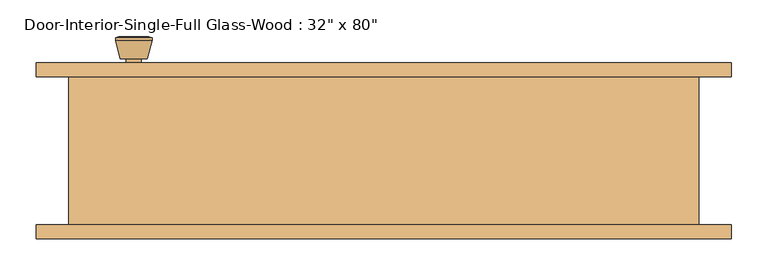
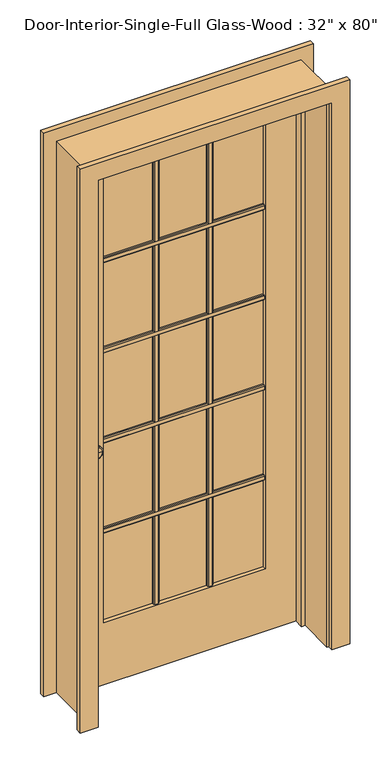
"""IFC4 building model written with IfcOpenShell, lengths in millimetres: door geometry."""

from ifc_helpers import new_model, si_unit, point, frame, frame_2d, origin, place, context, project, spatial, polyline, circle_curve, trimmed, segment, composite_curve, outline, extrude, faceted_brep, source, transform, mapped, element, save
from ifc_brep_helpers import plane_surface, cylinder_surface, revolved_surface, advanced_brep


def door_22967355(model_context):
    return source(origin(), model_context, "Body", "SolidModel", [
        extrude(outline(polyline([(84.455, 1586.23), (90.805, 1586.23), (93.98, 1583.055), (93.98, 1570.355), (90.805, 1567.18), (84.455, 1567.18), (84.455, 1586.23)])), frame((-285.75, 0.0, 0.0), z_axis=(1.0, 0.0, 0.0), x_axis=(0.0, 1.0, 0.0)), (0.0, 0.0, 1.0), 571.5),
        extrude(outline(polyline([(84.455, 1249.9975), (90.805, 1249.9975), (93.98, 1246.8225), (93.98, 1234.1225), (90.805, 1230.9475), (84.455, 1230.9475), (84.455, 1249.9975)])), frame((-285.75, 0.0, 0.0), z_axis=(1.0, 0.0, 0.0), x_axis=(0.0, 1.0, 0.0)), (0.0, 0.0, 1.0), 571.5),
        extrude(outline(polyline([(84.455, 913.765), (90.805, 913.765), (93.98, 910.59), (93.98, 897.89), (90.805, 894.715), (84.455, 894.715), (84.455, 913.765)])), frame((-285.75, 0.0, 0.0), z_axis=(1.0, 0.0, 0.0), x_axis=(0.0, 1.0, 0.0)), (0.0, 0.0, 1.0), 571.5),
        extrude(outline(polyline([(84.455, 577.5325), (90.805, 577.5325), (93.98, 574.3575), (93.98, 561.6575), (90.805, 558.4825), (84.455, 558.4825), (84.455, 577.5325)])), frame((-285.75, 0.0, 0.0), z_axis=(1.0, 0.0, 0.0), x_axis=(0.0, 1.0, 0.0)), (0.0, 0.0, 1.0), 571.5),
        extrude(outline(polyline([(85.725, 84.455), (85.725, 90.805), (88.9, 93.98), (101.6, 93.98), (104.775, 90.805), (104.775, 84.455), (85.725, 84.455)])), frame((0.0, 0.0, 231.775), z_axis=(0.0, 0.0, 1.0), x_axis=(1.0, 0.0, 0.0)), (0.0, 0.0, 1.0), 1681.1625),
        extrude(outline(polyline([(-104.775, 84.455), (-104.775, 90.805), (-101.6, 93.98), (-88.9, 93.98), (-85.725, 90.805), (-85.725, 84.455), (-104.775, 84.455)])), frame((0.0, 0.0, 231.775), z_axis=(0.0, 0.0, 1.0), x_axis=(1.0, 0.0, 0.0)), (0.0, 0.0, 1.0), 1681.1625),
        extrude(outline(polyline([(77.47, 1586.23), (77.47, 1567.18), (71.12, 1567.18), (67.945, 1570.355), (67.945, 1583.055), (71.12, 1586.23), (77.47, 1586.23)])), frame((-285.75, 0.0, 0.0), z_axis=(1.0, 0.0, 0.0), x_axis=(0.0, 1.0, 0.0)), (0.0, 0.0, 1.0), 571.5),
        extrude(outline(polyline([(77.47, 1249.9975), (77.47, 1230.9475), (71.12, 1230.9475), (67.945, 1234.1225), (67.945, 1246.8225), (71.12, 1249.9975), (77.47, 1249.9975)])), frame((-285.75, 0.0, 0.0), z_axis=(1.0, 0.0, 0.0), x_axis=(0.0, 1.0, 0.0)), (0.0, 0.0, 1.0), 571.5),
        extrude(outline(polyline([(77.47, 913.765), (77.47, 894.715), (71.12, 894.715), (67.945, 897.89), (67.945, 910.59), (71.12, 913.765), (77.47, 913.765)])), frame((-285.75, 0.0, 0.0), z_axis=(1.0, 0.0, 0.0), x_axis=(0.0, 1.0, 0.0)), (0.0, 0.0, 1.0), 571.5),
        extrude(outline(polyline([(77.47, 577.5325), (77.47, 558.4825), (71.12, 558.4825), (67.945, 561.6575), (67.945, 574.3575), (71.12, 577.5325), (77.47, 577.5325)])), frame((-285.75, 0.0, 0.0), z_axis=(1.0, 0.0, 0.0), x_axis=(0.0, 1.0, 0.0)), (0.0, 0.0, 1.0), 571.5),
        extrude(outline(polyline([(85.725, 77.47), (104.775, 77.47), (104.775, 71.12), (101.6, 67.945), (88.9, 67.945), (85.725, 71.12), (85.725, 77.47)])), frame((0.0, 0.0, 231.775), z_axis=(0.0, 0.0, 1.0), x_axis=(1.0, 0.0, 0.0)), (0.0, 0.0, 1.0), 1681.1625),
        extrude(outline(polyline([(-104.775, 77.47), (-85.725, 77.47), (-85.725, 71.12), (-88.9, 67.945), (-101.6, 67.945), (-104.775, 71.12), (-104.775, 77.47)])), frame((0.0, 0.0, 231.775), z_axis=(0.0, 0.0, 1.0), x_axis=(1.0, 0.0, 0.0)), (0.0, 0.0, 1.0), 1681.1625),
        advanced_brep(
        [(-342.9, 57.5, 914.4), (-332.9, 57.5, 914.4), (-352.9, 57.5, 914.4), (-322.4241324, 8.5, 914.4), (-342.9, 8.5, 914.4), (-363.3758676, 8.5, 914.4), (-317.9, 10.3278681, 914.4), (-367.9, 10.3278681, 914.4), (-317.9, 13.7915463, 914.4), (-367.9, 13.7915463, 914.4), (-324.263764, 38.5, 914.4), (-361.536236, 38.5, 914.4), (-332.9, 38.5, 914.4), (-352.9, 38.5, 914.4)],
        [
            (0, 1),
            (1, 2, circle_curve(frame((-342.9, 57.5, 914.4), z_axis=(0.0, 1.0, 0.0), x_axis=(-1.0, 0.0, 0.0)), 10.0)),
            (2, 0),
            (2, 1, circle_curve(frame((-342.9, 57.5, 914.4), z_axis=(0.0, 1.0, 0.0), x_axis=(-1.0, 0.0, 0.0)), 10.0)),
            (3, 4),
            (4, 5),
            (5, 3, circle_curve(frame((-342.9, 8.5, 914.4), z_axis=(0.0, -1.0, 0.0), x_axis=(-1.0, 0.0, 0.0)), 20.4758676)),
            (3, 5, circle_curve(frame((-342.9, 8.5, 914.4), z_axis=(0.0, -1.0, 0.0), x_axis=(-1.0, 0.0, 0.0)), 20.4758676)),
            (6, 3),
            (5, 7),
            (7, 6, circle_curve(frame((-342.9, 10.3278681, 914.4), z_axis=(0.0, -1.0, 0.0), x_axis=(-1.0, 0.0, 0.0)), 25.0)),
            (6, 7, circle_curve(frame((-342.9, 10.3278681, 914.4), z_axis=(0.0, -1.0, 0.0), x_axis=(-1.0, 0.0, 0.0)), 25.0)),
            (8, 6),
            (7, 9),
            (9, 8, circle_curve(frame((-342.9, 13.7915463, 914.4), z_axis=(0.0, -1.0, 0.0), x_axis=(-1.0, 0.0, 0.0)), 25.0)),
            (8, 9, circle_curve(frame((-342.9, 13.7915463, 914.4), z_axis=(0.0, -1.0, 0.0), x_axis=(-1.0, 0.0, 0.0)), 25.0)),
            (10, 8),
            (9, 11),
            (11, 10, circle_curve(frame((-342.9, 38.5, 914.4), z_axis=(0.0, -1.0, 0.0), x_axis=(-1.0, 0.0, 0.0)), 18.636236)),
            (10, 11, circle_curve(frame((-342.9, 38.5, 914.4), z_axis=(0.0, -1.0, 0.0), x_axis=(-1.0, 0.0, 0.0)), 18.636236)),
            (12, 10),
            (11, 13),
            (13, 12, circle_curve(frame((-342.9, 38.5, 914.4), z_axis=(0.0, -1.0, 0.0), x_axis=(-1.0, 0.0, 0.0)), 10.0)),
            (12, 13, circle_curve(frame((-342.9, 38.5, 914.4), z_axis=(0.0, -1.0, 0.0), x_axis=(-1.0, 0.0, 0.0)), 10.0)),
            (1, 12),
            (13, 2),
        ],
        [
            plane_surface(frame((-342.9, 57.5, 914.4), z_axis=(0.0, 1.0, 0.0), x_axis=(-1.0, 0.0, 0.0))),
            plane_surface(frame((-342.9, 8.5, 914.4), z_axis=(0.0, -1.0, 0.0), x_axis=(-1.0, 0.0, 0.0))),
            revolved_surface(polyline([(-363.3758676, 8.5, 914.4), (-367.9, 10.3278681, 914.4)]), (-342.9, 57.5, 914.4), (0.0, 1.0, 0.0)),
            cylinder_surface(frame((-342.9, 57.5, 914.4), z_axis=(0.0, 1.0, 0.0), x_axis=(-1.0, 0.0, 0.0)), 25.0),
            revolved_surface(polyline([(-367.9, 13.7915463, 914.4), (-361.536236, 38.5, 914.4)]), (-342.9, 57.5, 914.4), (0.0, 1.0, 0.0)),
            plane_surface(frame((-342.9, 38.5, 914.4), z_axis=(0.0, 1.0, 0.0), x_axis=(-1.0, 0.0, 0.0))),
            cylinder_surface(frame((-342.9, 57.5, 914.4), z_axis=(0.0, 1.0, 0.0), x_axis=(-1.0, 0.0, 0.0)), 10.0),
        ],
        [
            (0, [[1, 2, 3]]),
            (0, [[-3, 4, -1]]),
            (1, [[5, 6, 7]]),
            (1, [[-6, -5, 8]]),
            (2, [[9, -7, 10, 11]]),
            (2, [[-10, -8, -9, 12]]),
            (3, [[13, -11, 14, 15]]),
            (3, [[-14, -12, -13, 16]]),
            (4, [[17, -15, 18, 19]]),
            (4, [[-18, -16, -17, 20]]),
            (5, [[21, -19, 22, 23]]),
            (5, [[-22, -20, -21, 24]]),
            (6, [[25, -23, 26, -2]]),
            (6, [[-26, -24, -25, -4]]),
        ],
    ),
        extrude(outline(composite_curve([segment(trimmed(circle_curve(frame_2d((914.4, -342.9)), 30.0), [point((914.4, -372.9))], [point((914.4, -312.9))], False, "CARTESIAN"), True, "CONTINUOUS"), segment(trimmed(circle_curve(frame_2d((914.4, -342.9)), 30.0), [point((914.4, -312.9))], [point((914.4, -372.9))], False, "CARTESIAN"), True, "CONTINUOUS")], self_intersect=False)), frame((0.0, 57.5, 0.0), z_axis=(0.0, 1.0, 0.0), x_axis=(0.0, 0.0, 1.0)), (0.0, 0.0, 1.0), 6.0),
        advanced_brep(
        [(-342.9, 104.425, 914.4), (-352.9, 104.425, 914.4), (-332.9, 104.425, 914.4), (-322.4241324, 153.425, 914.4), (-363.3758676, 153.425, 914.4), (-342.9, 153.425, 914.4), (-317.9, 151.5971319, 914.4), (-367.9, 151.5971319, 914.4), (-317.9, 148.1334537, 914.4), (-367.9, 148.1334537, 914.4), (-324.263764, 123.425, 914.4), (-361.536236, 123.425, 914.4), (-332.9, 123.425, 914.4), (-352.9, 123.425, 914.4)],
        [
            (0, 1),
            (1, 2, circle_curve(frame((-342.9, 104.425, 914.4), z_axis=(0.0, -1.0, 0.0), x_axis=(-1.0, 0.0, 0.0)), 10.0)),
            (2, 0),
            (2, 1, circle_curve(frame((-342.9, 104.425, 914.4), z_axis=(0.0, -1.0, 0.0), x_axis=(-1.0, 0.0, 0.0)), 10.0)),
            (3, 4, circle_curve(frame((-342.9, 153.425, 914.4), z_axis=(0.0, 1.0, 0.0), x_axis=(-1.0, 0.0, 0.0)), 20.4758676)),
            (4, 5),
            (5, 3),
            (4, 3, circle_curve(frame((-342.9, 153.425, 914.4), z_axis=(0.0, 1.0, 0.0), x_axis=(-1.0, 0.0, 0.0)), 20.4758676)),
            (6, 7, circle_curve(frame((-342.9, 151.5971319, 914.4), z_axis=(0.0, 1.0, 0.0), x_axis=(-1.0, 0.0, 0.0)), 25.0)),
            (7, 4),
            (3, 6),
            (7, 6, circle_curve(frame((-342.9, 151.5971319, 914.4), z_axis=(0.0, 1.0, 0.0), x_axis=(-1.0, 0.0, 0.0)), 25.0)),
            (8, 9, circle_curve(frame((-342.9, 148.1334537, 914.4), z_axis=(0.0, 1.0, 0.0), x_axis=(-1.0, 0.0, 0.0)), 25.0)),
            (9, 7),
            (6, 8),
            (9, 8, circle_curve(frame((-342.9, 148.1334537, 914.4), z_axis=(0.0, 1.0, 0.0), x_axis=(-1.0, 0.0, 0.0)), 25.0)),
            (10, 11, circle_curve(frame((-342.9, 123.425, 914.4), z_axis=(0.0, 1.0, 0.0), x_axis=(-1.0, 0.0, 0.0)), 18.636236)),
            (11, 9),
            (8, 10),
            (11, 10, circle_curve(frame((-342.9, 123.425, 914.4), z_axis=(0.0, 1.0, 0.0), x_axis=(-1.0, 0.0, 0.0)), 18.636236)),
            (12, 13, circle_curve(frame((-342.9, 123.425, 914.4), z_axis=(0.0, 1.0, 0.0), x_axis=(-1.0, 0.0, 0.0)), 10.0)),
            (13, 11),
            (10, 12),
            (13, 12, circle_curve(frame((-342.9, 123.425, 914.4), z_axis=(0.0, 1.0, 0.0), x_axis=(-1.0, 0.0, 0.0)), 10.0)),
            (1, 13),
            (12, 2),
        ],
        [
            plane_surface(frame((-342.9, 104.425, 914.4), z_axis=(0.0, -1.0, 0.0), x_axis=(-1.0, 0.0, 0.0))),
            plane_surface(frame((-342.9, 153.425, 914.4), z_axis=(0.0, 1.0, 0.0), x_axis=(-1.0, 0.0, 0.0))),
            revolved_surface(polyline([(-363.3758676, 153.425, 914.4), (-367.9, 151.5971319, 914.4)]), (-342.9, 104.425, 914.4), (0.0, -1.0, 0.0)),
            cylinder_surface(frame((-342.9, 104.425, 914.4), z_axis=(0.0, -1.0, 0.0), x_axis=(-1.0, 0.0, 0.0)), 25.0),
            revolved_surface(polyline([(-367.9, 148.1334537, 914.4), (-361.536236, 123.425, 914.4)]), (-342.9, 104.425, 914.4), (0.0, -1.0, 0.0)),
            plane_surface(frame((-342.9, 123.425, 914.4), z_axis=(0.0, -1.0, 0.0), x_axis=(-1.0, 0.0, 0.0))),
            cylinder_surface(frame((-342.9, 104.425, 914.4), z_axis=(0.0, -1.0, 0.0), x_axis=(-1.0, 0.0, 0.0)), 10.0),
        ],
        [
            (0, [[1, 2, 3]]),
            (0, [[-3, 4, -1]]),
            (1, [[5, 6, 7]]),
            (1, [[8, -7, -6]]),
            (2, [[9, 10, -5, 11]]),
            (2, [[12, -11, -8, -10]]),
            (3, [[13, 14, -9, 15]]),
            (3, [[16, -15, -12, -14]]),
            (4, [[17, 18, -13, 19]]),
            (4, [[20, -19, -16, -18]]),
            (5, [[21, 22, -17, 23]]),
            (5, [[24, -23, -20, -22]]),
            (6, [[-2, 25, -21, 26]]),
            (6, [[-4, -26, -24, -25]]),
        ],
    ),
        extrude(outline(composite_curve([segment(trimmed(circle_curve(frame_2d((914.4, -342.9)), 30.0), [point((914.4, -372.9))], [point((914.4, -312.9))], False, "CARTESIAN"), True, "CONTINUOUS"), segment(trimmed(circle_curve(frame_2d((914.4, -342.9)), 30.0), [point((914.4, -312.9))], [point((914.4, -372.9))], False, "CARTESIAN"), True, "CONTINUOUS")], self_intersect=False)), frame((0.0, 98.425, 0.0), z_axis=(0.0, 1.0, 0.0), x_axis=(0.0, 0.0, 1.0)), (0.0, 0.0, 1.0), 6.0),
        extrude(outline(polyline([(2032.0, -406.4), (0.0, -406.4), (0.0, 406.4), (2032.0, 406.4), (2032.0, -406.4)]), holes=[polyline([(1912.9375, -285.75), (1912.9375, 285.75), (231.775, 285.75), (231.775, -285.75), (1912.9375, -285.75)])]), frame((0.0, 63.5, 0.0), z_axis=(0.0, 1.0, 0.0), x_axis=(0.0, 0.0, 1.0)), (0.0, 0.0, 1.0), 34.925),
        faceted_brep([(431.8, 98.425, 0.0), (431.8, -104.775, 0.0), (406.4, -104.775, 0.0), (406.4, 28.575, 0.0), (393.7, 28.575, 0.0), (393.7, 63.5, 0.0), (406.4, 63.5, 0.0), (406.4, 98.425, 0.0), (431.8, 98.425, 2057.4), (431.8, -104.775, 2057.4), (-431.8, -104.775, 2057.4), (-431.8, -104.775, 0.0), (-406.4, -104.775, 0.0), (-406.4, -104.775, 2032.0), (406.4, -104.775, 2032.0), (406.4, 28.575, 2032.0), (-406.4, 28.575, 2032.0), (-406.4, 28.575, 0.0), (-393.7, 28.575, 0.0), (-393.7, 28.575, 2019.3), (393.7, 28.575, 2019.3), (393.7, 63.5, 2019.3), (-393.7, 63.5, 2019.3), (-393.7, 63.5, 0.0), (-406.4, 63.5, 0.0), (-406.4, 63.5, 2032.0), (406.4, 63.5, 2032.0), (406.4, 98.425, 2032.0), (-406.4, 98.425, 2032.0), (-406.4, 98.425, 0.0), (-431.8, 98.425, 0.0), (-431.8, 98.425, 2057.4)], [[[0, 1, 2, 3, 4, 5, 6, 7]], [[1, 0, 8, 9]], [[2, 1, 9, 10, 11, 12, 13, 14]], [[3, 2, 14, 15]], [[4, 3, 15, 16, 17, 18, 19, 20]], [[5, 4, 20, 21]], [[6, 5, 21, 22, 23, 24, 25, 26]], [[7, 6, 26, 27]], [[0, 7, 27, 28, 29, 30, 31, 8]], [[9, 8, 31, 10]], [[15, 14, 13, 16]], [[21, 20, 19, 22]], [[27, 26, 25, 28]], [[30, 29, 24, 23, 18, 17, 12, 11]], [[10, 31, 30, 11]], [[16, 13, 12, 17]], [[22, 19, 18, 23]], [[28, 25, 24, 29]]]),
        extrude(outline(polyline([(285.75, 77.47), (-285.75, 77.47), (-285.75, 84.455), (285.75, 84.455), (285.75, 77.47)])), frame((0.0, 0.0, 231.775), z_axis=(0.0, 0.0, 1.0), x_axis=(1.0, 0.0, 0.0)), (0.0, 0.0, 1.0), 1681.1625),
        extrude(outline(polyline([(0.0, 412.75), (0.0, 476.25), (2101.85, 476.25), (2101.85, -476.25), (0.0, -476.25), (0.0, -412.75), (2038.35, -412.75), (2038.35, 412.75), (0.0, 412.75)])), frame((0.0, -123.825, 0.0), z_axis=(0.0, 1.0, 0.0), x_axis=(0.0, 0.0, 1.0)), (0.0, 0.0, 1.0), 19.05),
        extrude(outline(polyline([(0.0, 412.75), (0.0, 476.25), (2101.85, 476.25), (2101.85, -476.25), (0.0, -476.25), (0.0, -412.75), (2038.35, -412.75), (2038.35, 412.75), (0.0, 412.75)])), frame((0.0, 98.425, 0.0), z_axis=(0.0, 1.0, 0.0), x_axis=(0.0, 0.0, 1.0)), (0.0, 0.0, 1.0), 19.05),
    ])


if __name__ == "__main__":
    model = new_model("IFC4")
    model_context = context("Model", 3, world=origin())
    ifc_project = project(units=[si_unit("LENGTHUNIT", "METRE", prefix="MILLI")], contexts=[model_context])
    site = spatial("IfcSite", under=ifc_project)
    building = spatial("IfcBuilding", under=site)
    placement = place(None, origin())
    door_shape = door_22967355(model_context)
    element("IfcDoor", 1, ObjectType="Door-Interior-Single-Full Glass-Wood : 32\" x 80\"", at=placement, inside=building, context=model_context, shape_type="MappedRepresentation", body=[
        mapped(door_shape, transform((0.0, 0.0, 0.0), x_axis=(1.0, 0.0, 0.0), y_axis=(0.0, 1.0, 0.0), z_axis=(0.0, 0.0, 1.0))),
    ])
    save(model, "model.ifc")

# Revit data of these elements
# Type "Door-Interior-Single-Full Glass-Wood : 32\" x 80\""
#   Type Mark = "10"
#   Assembly Code = "C1020300"
#   Analytic Construction = "Wood frame with single clear glass"
#   Top Rail = 0' - 4 11/16"
#   Thickness = 0' - 1 3/8"
#   Thermal Resistance (R) = 1.0102 (h·ft²·°F)/BTU
#   Swing Angle [instance default] = 90.00°
#   Stiles = 0' - 4 3/4"
#   Rough Width = 2' - 10"
#   Rough Height = 6' - 9"
#   Height = 6' - 8"
#   Width = 2' - 8"
#   Heat Transfer Coefficient (U) = 0.9900 BTU/(h·ft²·°F)
#   Bottom Rail = 0' - 9 1/8"
#   Show Grill [instance default] = yes
#   Trim Material = Cherry
#   Panel Material = Cherry
#   Frame Material = Cherry
#   Door Handle Material = Aluminum
#   Visual Light Transmittance = 0
#   Solar Heat Gain Coefficient = 0
#   Wall Closure = (empty or 0)
#   Function = (empty or 0)
# Element 1 (IfcDoor, "Door-Interior-Single-Full Glass-Wood : 32\" x 80\"")
#   Materials on its faces: "Cherry", "Aluminum", "Glass"
# Materials
#   "Cherry": class "Wood", colour RGB 226 177 128, transparency 0, Description = "Prunus Serotina", Cost = 0
#   "Aluminum": class "Metal", colour RGB 247 247 247, transparency 0, Description = "Aluminum 6061", Cost = 0
#   "Glass": class "Glass", colour RGB 0 128 192, transparency 0.75, Description = "Soda Lime Glass", Cost = 0
